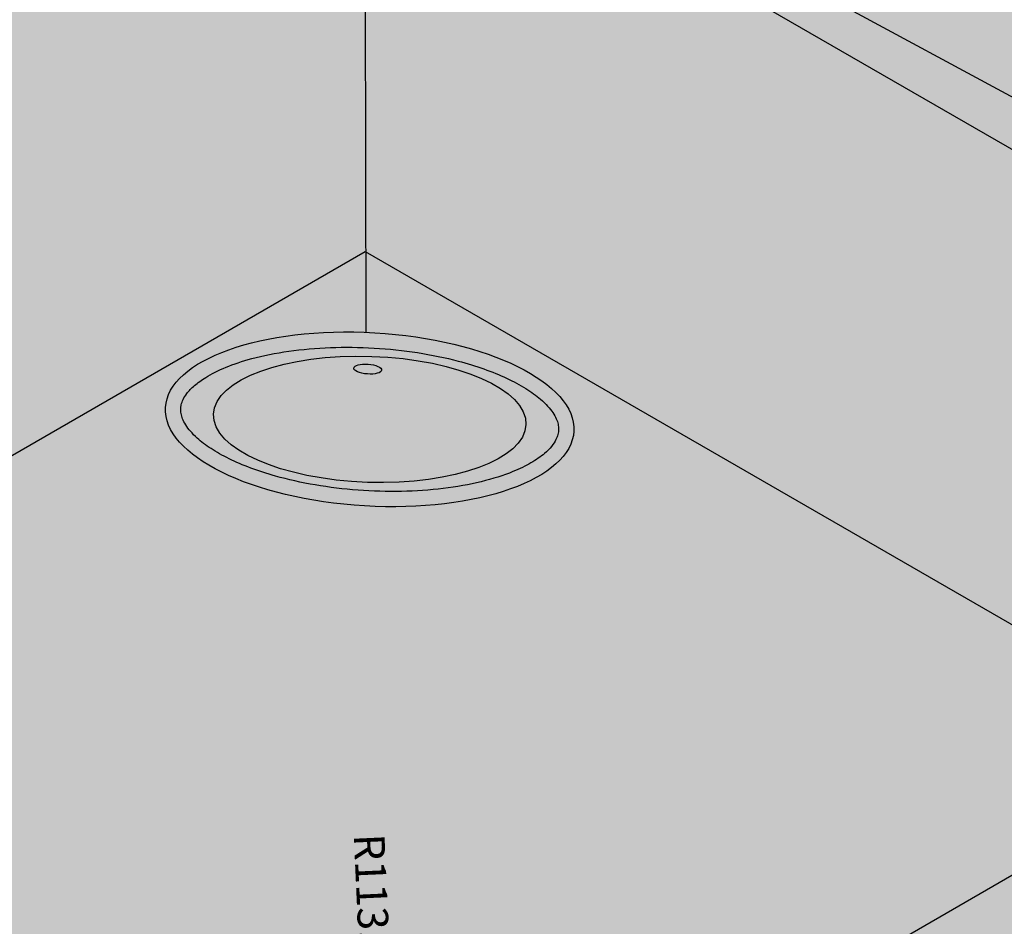
# Model space of a CAD drawing. Units: millimetres. Extents: x 78378 to 86415, y 148682 to 152721.
# Tile 13 of 18: x 80164 to 80806, y 150495 to 151086. Entities that reach past the tile are written whole.
import ezdxf

# ---------------------------------------------------------------- set-up
doc = ezdxf.new("R2010")
doc.units = ezdxf.units.MM
for name, color, linetype, lineweight in [('A-ANNO-DIMS', 2, 'Continuous', 18), ('A-FURN', 4, 'Continuous', 25), ('A-FURN-PATT', 32, 'Continuous', 13)]:
    doc.layers.add(name, color=color, linetype=linetype, lineweight=lineweight)
doc.styles.get("Standard").update_dxf_attribs({"font": 'arial.ttf'})
doc.dimstyles.new('ISO-25', dxfattribs={"dimtxt": 20, "dimasz": 20, "dimexe": 1.25, "dimexo": 0.625, "dimtad": 0, "dimdec": 1, "dimtxsty": 'Standard', "dimcen": 2.5, "dimadec": 0, "dimazin": 0, "dimtfac": 1, "dimtdec": 1, "dimtmove": 0, "dimatfit": 3, "dimfxl": 1, "dimarcsym": 0})

# ---------------------------------------------------------------- blocks, each defined once
blk = doc.blocks.new('*D65')
at = {"layer": 'A-ANNO-DIMS', "color": 0, "lineweight": -2, "transparency": 16777216}
for p, q in [((80394.08, 150453.29), (80394.98, 150433.31)), ((80401.02, 150300.38), (80395.89, 150413.33))]:
    blk.add_line(p, q, dxfattribs=at)
at = {"layer": 'A-ANNO-DIMS', "color": 0, "transparency": 16777216}
blk.add_solid([(80398.31, 150433.46), (80391.65, 150433.16), (80395.89, 150413.33)], dxfattribs=at)
at = {"layer": 'Defpoints', "color": 0, "transparency": 16777216}
for p in [(80395.89, 150413.33), (80401.02, 150300.38)]:
    blk.add_point(p, dxfattribs=at)
at = {"layer": 'A-ANNO-DIMS', "color": 0, "transparency": 16777216, "insert": (80391.73, 150504.94), "char_height": 20, "attachment_point": 5, "rotation": 272.60064}
blk.add_mtext('R113.06', dxfattribs=at)

msp = doc.modelspace()

# ---------------------------------------------------------------- hatches: boundary and pattern name
at = {"layer": 'A-FURN-PATT'}
h = msp.add_hatch(color=256, dxfattribs=at)
h.dxf.hatch_style = 1
h.paths.add_polyline_path([(78839.3276, 151040.0076), (78579.52, 151190.0076), (78579.52, 150470.0076), (78839.3276, 150320.0076)])
h.paths.add_polyline_path([(79073.1545, 150899.6469, 0.27777969), (79002.2645, 150996.3205, 0.79108393), (78917.9567, 150978.8719, 0.18044832), (78856.6481, 150853.0138), (78856.6481, 150350.6973), (79073.1545, 150484.318)])
h.paths.add_polyline_path([(79073.1545, 151175.0076), (78856.6481, 151050.0076), (78856.6481, 150853.0138, -0.18044832), (78917.9567, 150978.8719, -0.79108393), (79002.2645, 150996.3205, -0.27777969), (79073.1545, 150899.6469)])
h.paths.add_polyline_path([(79341.6224, 151350.0076), (79099.1352, 151490.0076), (78596.8405, 151200.0076), (78839.3276, 151060.0076)])
h.paths.add_polyline_path([(79904.5389, 151675.0076), (79662.0518, 151815.0076), (79099.1352, 151490.0076), (79341.6224, 151350.0076)])
h.paths.add_polyline_path([(80389.5131, 151955.0076), (80389.5131, 152235.0076), (79662.0518, 151815.0076), (79904.5389, 151675.0076)])
h.paths.add_polyline_path([(80389.5131, 151955.0076), (80164.3465, 151825.0076), (80164.3465, 151105.0076), (80614.6797, 151105.0076), (80614.6797, 151825.0076)])
edge = h.paths.add_edge_path(flags=16)
edge.add_spline(control_points=[(80216.308, 151728.251), (80227.1854, 151732.981), (80256.3301, 151745.6544), (80298.41, 151761.9595), (80340.2597, 151805.855), (80391.0771, 151782.0404), (80454.0396, 151805.7581), (80496.5007, 151742.4095), (80543.8218, 151733.4043), (80562.7182, 151729.8083)], knot_values=[0, 0, 0, 0, 35.54374676, 95.23575347, 136.36767513, 200.93298197, 236.72641081, 322.88993498, 380.17027367, 380.17027367, 380.17027367, 380.17027367], degree=3, periodic=0)
edge.add_line((80562.7182, 151729.8083), (80562.7182, 151165.0076))
edge.add_line((80562.7182, 151165.0076), (80216.308, 151165.0076))
edge.add_line((80216.308, 151165.0076), (80216.308, 151728.251))
h.paths.add_polyline_path([(80632.0002, 152095.0076), (80389.5131, 152235.0076), (80389.5131, 151955.0076), (80614.6797, 151825.0076), (80632.0002, 151815.0076)])
h.paths.add_polyline_path([(80867.7794, 151958.8805), (80632.0002, 152095.0076), (80632.0002, 151815.0076), (80632.0002, 151510.0076), (80867.7794, 151373.8805)])
h.paths.add_polyline_path([(80147.026, 151495.8203, 0.18918979), (80063.5671, 151597.7244, 0.78826136), (79979.2691, 151580.5832, 0.16072613), (79904.5389, 151413.5769), (79904.5389, 150955.0076), (80147.026, 151095.0076)])
h.paths.add_polyline_path([(80147.026, 151815.0076), (79904.5389, 151675.0076), (79904.5389, 151413.5769, -0.16072613), (79979.2691, 151580.5832, -0.78826136), (80063.5671, 151597.7244, -0.18918979), (80147.026, 151495.8203)])
h.paths.add_polyline_path([(79887.2184, 151645.0076), (79640.4011, 151502.5076), (79640.4011, 151262.3325, -0.16072613), (79715.1313, 151429.3387, -0.78826136), (79799.4294, 151446.48, -0.21290578), (79887.2184, 151328.7247)])
h.paths.add_polyline_path([(79799.4294, 151446.48, 0.78826136), (79715.1313, 151429.3387, 0.16072613), (79640.4011, 151262.3325), (79640.4011, 150822.5076), (79887.2184, 150965.0076), (79887.2184, 151328.7247, 0.21290578)])
h.paths.add_polyline_path([(79605.7601, 151482.5076), (79358.9429, 151340.0076), (79358.9429, 151100.0701, -0.16072613), (79433.6731, 151267.0764, -0.78826136), (79517.9711, 151284.2176, -0.21290578), (79605.7601, 151166.4623)])
h.paths.add_polyline_path([(79605.7601, 151166.4623, 0.21290578), (79517.9711, 151284.2176, 0.78826136), (79433.6731, 151267.0764, 0.16072613), (79358.9429, 151100.0701), (79358.9429, 150742.9831), (79419.0877, 150694.7323), (79605.7601, 150802.5076)])
edge = h.paths.add_edge_path(flags=0)
edge.add_spline(control_points=[(81152.4356, 151098.7676), (81105.7208, 151145.9466), (81038.6136, 151213.7208), (80882.3866, 151214.1938), (80797.4434, 151311.2997), (80711.8686, 151340.3754), (80681.7691, 151350.6023)], knot_values=[0, 0, 0, 0, 188.233441, 270.4032752, 445.45179201, 540.42858829, 540.42858829, 540.42858829, 540.42858829], degree=3, periodic=0)
edge.add_line((80683.4538, 151350.0269), (80683.4538, 151104.8792))
edge.add_line((80683.4538, 151104.8792), (81152.4356, 150851.399))
edge.add_line((81152.4356, 150851.399), (81152.4356, 151098.7676))
edge = h.paths.add_edge_path(flags=0)
edge.add_spline(control_points=[(80912.9018, 151027.1103), (80892.3742, 151034.1027), (80860.1663, 151045.0739), (80835.5097, 151068.1214), (80826.5679, 151076.4797)], knot_values=[0, 0, 0, 0, 63.98405104, 100.39142428, 100.39142428, 100.39142428, 100.39142428], degree=3, periodic=0)
edge.add_arc((80830.0414, 151081.2992), 5.9407, 100.9277276, 234.2187381, ccw=False)
edge.add_spline(control_points=[(80828.9152, 151087.1322), (80837.857, 151078.7739), (80862.5136, 151055.7263), (80894.7215, 151044.7552), (80915.2491, 151037.7628)], knot_values=[0, 0, 0, 0, 36.40737324, 100.39142428, 100.39142428, 100.39142428, 100.39142428], degree=3, periodic=0)
edge.add_arc((80914.7882, 151032.2795), 5.5026, -107.9540399, 85.195579, ccw=False)
h.paths.add_polyline_path([(81238.218, 151110.0076), (80632.0002, 151460.0076), (80632.0002, 151105.0076), (81238.218, 150755.0076)])
edge = h.paths.add_edge_path(flags=16)
edge.add_line((81152.4356, 150851.399), (80683.4538, 151104.8792))
edge.add_line((80683.4538, 151104.8792), (80683.4538, 151350.0279))
edge.add_spline(control_points=[(80681.7691, 151350.6023), (80711.8686, 151340.3754), (80797.4434, 151311.2997), (80882.3866, 151214.1938), (81038.6136, 151213.7208), (81105.7208, 151145.9466), (81152.4356, 151098.7676)], knot_values=[0, 0, 0, 0, 94.97679628, 270.02531309, 352.19514729, 540.42858829, 540.42858829, 540.42858829, 540.42858829], degree=3, periodic=0)
edge.add_line((81152.4356, 151098.7676), (81152.4356, 150851.399))
edge = h.paths.add_edge_path(flags=0)
edge.add_spline(control_points=[(80912.9018, 151027.1103), (80892.3742, 151034.1027), (80860.1663, 151045.0739), (80835.5097, 151068.1214), (80826.5679, 151076.4797)], knot_values=[0, 0, 0, 0, 63.98405104, 100.39142428, 100.39142428, 100.39142428, 100.39142428], degree=3, periodic=0)
edge.add_arc((80830.0414, 151081.2992), 5.9407, 100.9277276, 234.2187381, ccw=False)
edge.add_spline(control_points=[(80828.9152, 151087.1322), (80837.857, 151078.7739), (80862.5136, 151055.7263), (80894.7215, 151044.7552), (80915.2491, 151037.7628)], knot_values=[0, 0, 0, 0, 36.40737324, 100.39142428, 100.39142428, 100.39142428, 100.39142428], degree=3, periodic=0)
edge.add_arc((80914.7882, 151032.2795), 5.5026, -107.7417882, 85.195579, ccw=False)
h.paths.add_polyline_path([(81498.0256, 151255.0076), (81238.218, 151110.0076), (81238.218, 150755.0076), (81498.0256, 150905.0076)])
edge = h.paths.add_edge_path(flags=16)
edge.add_spline(control_points=[(81152.4356, 151098.7676), (81105.7208, 151145.9466), (81038.6136, 151213.7208), (80882.3866, 151214.1938), (80797.4434, 151311.2997), (80711.8686, 151340.3754), (80681.7691, 151350.6023)], knot_values=[0, 0, 0, 0, 188.233441, 270.4032752, 445.45179201, 540.42858829, 540.42858829, 540.42858829, 540.42858829], degree=3, periodic=0)
edge.add_line((80683.4538, 151350.0279), (80683.4538, 151104.8792))
edge.add_line((80683.4538, 151104.8792), (81152.4356, 150851.399))
edge.add_line((81152.4356, 150851.399), (81152.4356, 151098.7676))
h.paths.add_polyline_path([(81453.9904, 151280.4314), (80867.7794, 151618.8805), (80867.7794, 151373.8805), (81238.218, 151160.0076)])
edge = h.paths.add_edge_path(flags=16)
edge.add_line((81189.2304, 151297.6373), (81114.4166, 151300.2154))
edge.add_arc((81412.0967, 151394.0167), 312.1092, 179.7569303, 197.4900342, ccw=False)
edge.add_ellipse((81154.0183, 151392.0436), major_axis=(-54.0264, 3.6301), ratio=0.22179693, start_angle=0, end_angle=0.3517985, ccw=False)
edge.add_ellipse((81154.0183, 151392.0436), major_axis=(-54.0264, 3.6301), ratio=0.22179693, start_angle=180, end_angle=360, ccw=False)
edge.add_spline(control_points=[(81196.1844, 151321.9476), (81224.9802, 151347.1455), (81266.8846, 151383.8144), (81222.0354, 151387.0304), (81208.0056, 151388.0364)], knot_values=[0, 0, 0, 0, 75.09175173, 109.27580439, 109.27580439, 109.27580439, 109.27580439], degree=3, periodic=0)
edge.add_arc((80751.9112, 151435.6145), 458.5693, 342.4891602, 345.646172, ccw=False)
edge = h.paths.add_edge_path(flags=0)
edge.add_spline(control_points=[(81196.6193, 151323.657), (81197.893, 151324.7717), (81199.1654, 151325.8858), (81209.0233, 151334.5343), (81217.3959, 151341.9835), (81228.0928, 151352.5012), (81231.3883, 151355.9524), (81236.9493, 151362.4395), (81239.214, 151365.4773), (81241.4987, 151369.416), (81242.064, 151370.5542), (81242.9187, 151372.6971), (81243.2076, 151373.7015), (81243.5012, 151375.5539), (81243.5065, 151376.4), (81243.2432, 151377.9407), (81242.9775, 151378.6373), (81242.1402, 151379.937), (81241.5659, 151380.5416), (81240.2039, 151381.533), (81239.4963, 151381.9384), (81237.0619, 151383.0663), (81235.0242, 151383.6999), (81230.352, 151384.7569), (81227.7173, 151385.1826), (81221.9118, 151385.9145), (81218.7193, 151386.2133), (81213.7912, 151386.6115), (81212.1252, 151386.7359), (81209.6196, 151386.9181), (81208.7865, 151386.9779), (81207.9009, 151387.0432)], knot_values=[0.01548744, 0.01548744, 0.01548744, 0.01548744, 3.33787957, 3.33787957, 25.85130624, 25.85130624, 37.52811308, 37.52811308, 49.20491992, 49.20491992, 54.2850938, 54.2850938, 59.36526768, 59.36526768, 64.44544157, 64.44544157, 69.52561545, 69.52561545, 74.60578933, 74.60578933, 78.49366785, 78.49366785, 86.25567095, 86.25567095, 94.01767406, 94.01767406, 102.20226556, 102.20226556, 106.29456131, 106.29456131, 108.32522175, 108.32522175, 108.32522175, 108.32522175], degree=3, periodic=0)
edge = h.paths.add_edge_path(flags=16)
edge.add_arc((81034.1732, 151350.4693), 42.5822, 231.2679035, 306.151846, ccw=False)
edge.add_line((81007.5303, 151317.2517), (81007.5303, 151395.181))
edge.add_ellipse((81033.412, 151394.7791), major_axis=(-25.8816, 0.4538), ratio=0.23894509, start_angle=0, end_angle=0.1147075, ccw=False)
edge.add_ellipse((81033.412, 151394.7791), major_axis=(-25.8816, 0.4538), ratio=0.23894509, start_angle=181.1677709, end_angle=358.9476457, ccw=False)
edge.add_ellipse((81033.412, 151395.7791), major_axis=(-25.8816, 0.4538), ratio=0.23894509, start_angle=180, end_angle=360.1147075, ccw=False)
edge.add_ellipse((81033.412, 151395.7791), major_axis=(-25.8816, 0.4538), ratio=0.23894509, start_angle=178.9476457, end_angle=180, ccw=False)
edge.add_line((81059.2936, 151395.1778), (81059.2936, 151394.3772))
edge.add_ellipse((81033.412, 151394.7791), major_axis=(-25.8816, 0.4538), ratio=0.23894509, start_angle=180, end_angle=180.1147075, ccw=False)
edge.add_ellipse((81033.412, 151394.7791), major_axis=(-25.8816, 0.4538), ratio=0.23894509, start_angle=3.6903098, end_angle=176.4406503, ccw=False)
edge.add_line((81059.2936, 151393.3388), (81059.2936, 151316.086))
h.paths.add_polyline_path([(80951.9355, 151343.9568), (80909.6838, 151362.4635), (80904.0219, 151443.9615, -0.38133308), (80987.2169, 151411.3717)], flags=16)
h = msp.add_hatch(color=256, dxfattribs=at)
h.dxf.hatch_style = 1
h.paths.add_polyline_path([(80389.8136, 150935.1811), (80389.5131, 151105.0076), (80164.3465, 151105.0076), (79904.5389, 150955.0076), (79433.5848, 150683.1022), (79459.4128, 150662.3818), (79243.9048, 150537.9582), (79160.4069, 150518.1674), (78839.3276, 150320.0076), (78579.52, 150470.0076), (78570.8597, 150475.0076), (78570.8597, 150465.0076), (78570.8597, 149885.0076)])
h.paths.add_polyline_path([(80086.4042, 150460.0076), (79826.5966, 150610.0076), (78570.8597, 149885.0076), (78830.6674, 149735.0076)])
h.paths.add_polyline_path([(79540.8001, 150161.0557), (79217.3967, 149974.3386), (78980.9166, 150110.8705), (79304.32, 150297.5875)], flags=16)
h.paths.add_polyline_path([(79506.159, 150161.0557), (79217.3967, 149994.3386), (79015.5576, 150110.8705), (79304.32, 150277.5875)], flags=0)
edge = h.paths.add_edge_path(flags=0)
edge.add_arc((79247.8636, 150177.1541), 137.9799, 256.0025928, 293.5594109)
edge.add_arc((79240.7671, 150078.2605), 68.0855, 336.099104, 387.3696877)
edge.add_ellipse((79258.3074, 150109.4852), major_axis=(-42.6234, -1.6591), ratio=0.16042843, start_angle=0, end_angle=179.0977279, ccw=False)
edge.add_arc((79285.2112, 150074.2509), 77.2096, 155.1233104, 203.6557939)
edge = h.paths.add_edge_path(flags=0)
edge.add_ellipse((79258.6958, 150110.8297), major_axis=(-42.6234, -1.6591), ratio=0.16042843, start_angle=350.6039412, end_angle=356.2289762)
edge.add_line((79219.169, 150111.8937), (79218.3268, 150109.4141))
edge.add_arc((79262.4675, 150032.9602), 88.2813, 112.3931229, 120, ccw=False)
h.paths.add_polyline_path([(79287.0625, 150086.9703, -0.24770206), (79288.1967, 150077.2955, -0.39047651), (79265.4731, 150072.5438, -0.48726153), (79264.079, 150082.3769, 0.39560433)], flags=0)
h.paths.add_polyline_path([(80389.5131, 150935.0076), (79826.5966, 150610.0076), (80086.4042, 150460.0076), (80692.622, 150460.0076), (80952.4296, 150610.0076)])
edge = h.paths.add_edge_path(flags=16)
edge.add_ellipse((80392.4466, 150825.601), major_axis=(-133.0757, 7.722), ratio=0.42449957, start_angle=0, end_angle=360)
edge = h.paths.add_edge_path(flags=0)
edge.add_spline(control_points=[(80269.3541, 150832.7436), (80269.2919, 150831.672), (80269.3503, 150830.5922), (80269.7341, 150828.3361), (80270.0612, 150827.1587), (80271.0461, 150824.6748), (80271.7052, 150823.3692), (80273.4061, 150820.6503), (80274.4481, 150819.2381), (80276.9366, 150816.3509), (80278.3828, 150814.8762), (80282.5858, 150811.0913), (80285.6261, 150808.7701), (80292.6031, 150804.2267), (80296.5388, 150802.0041), (80305.195, 150797.7581), (80309.9151, 150795.7344), (80320.0112, 150791.96), (80325.387, 150790.2092), (80339.2162, 150786.315), (80347.9578, 150784.3563), (80366.0679, 150781.2568), (80375.4359, 150780.1158), (80394.3093, 150778.7158), (80403.8142, 150778.4568), (80422.4656, 150778.8319), (80431.6115, 150779.4662), (80449.0608, 150781.5838), (80457.3636, 150783.0675), (80472.6699, 150786.7766), (80479.6726, 150789.0033), (80490.1894, 150793.2813), (80494.1268, 150795.1967), (80501.0146, 150799.1885), (80503.9632, 150801.2651), (80508.2066, 150804.9015), (80509.73, 150806.4609), (80512.1996, 150809.4942), (80513.1456, 150810.9657), (80514.4291, 150813.5431), (80514.8436, 150814.6688), (80515.3984, 150816.8625), (80515.5405, 150817.9315), (80515.5801, 150820.098), (80515.4773, 150821.1978), (80514.9905, 150823.5062), (80514.6047, 150824.7154), (80513.4854, 150827.2641), (80512.7511, 150828.6027), (80510.8872, 150831.3809), (80509.7578, 150832.8196), (80507.0873, 150835.7513), (80505.5466, 150837.2439), (80501.0624, 150841.0944), (80497.8199, 150843.4576), (80490.4174, 150848.062), (80486.2582, 150850.3037), (80477.1448, 150854.5643), (80472.1909, 150856.5835), (80461.6275, 150860.3245), (80456.0182, 150862.0465), (80441.7332, 150865.8127), (80432.7885, 150867.6675), (80414.3391, 150870.5317), (80404.8349, 150871.5411), (80385.7707, 150872.6572), (80376.2113, 150872.764), (80357.5444, 150872.0728), (80348.4375, 150871.2748), (80331.1682, 150868.83), (80323.0064, 150867.1827), (80309.472, 150863.5363), (80303.8628, 150861.6593), (80293.8018, 150857.5401), (80289.3512, 150855.2969), (80282.7757, 150851.2345), (80280.3473, 150849.4579), (80276.2606, 150845.9127), (80274.604, 150844.1458), (80272.3157, 150841.1243), (80271.5358, 150839.8454), (80270.3496, 150837.3879), (80269.9417, 150836.2101), (80269.5065, 150834.2815), (80269.3988, 150833.5143), (80269.3541, 150832.7436)], knot_values=[0, 0, 0, 0, 0.09750046, 0.09750046, 0.19500092, 0.19500092, 0.29250138, 0.29250138, 0.39000184, 0.39000184, 0.4875023, 0.4875023, 0.63880322, 0.63880322, 0.79010415, 0.79010415, 0.94140507, 0.94140507, 1.092706, 1.092706, 1.3128171, 1.3128171, 1.5329282, 1.5329282, 1.7530393, 1.7530393, 1.97315041, 1.97315041, 2.19326151, 2.19326151, 2.41337261, 2.41337261, 2.56986063, 2.56986063, 2.72634866, 2.72634866, 2.84418658, 2.84418658, 2.96202451, 2.96202451, 3.06023388, 3.06023388, 3.15844325, 3.15844325, 3.25665261, 3.25665261, 3.35486198, 3.35486198, 3.45307135, 3.45307135, 3.55128072, 3.55128072, 3.64949009, 3.64949009, 3.80392773, 3.80392773, 3.95836537, 3.95836537, 4.11280301, 4.11280301, 4.26724064, 4.26724064, 4.48920349, 4.48920349, 4.71116635, 4.71116635, 4.9331292, 4.9331292, 5.15509205, 5.15509205, 5.3770549, 5.3770549, 5.55785361, 5.55785361, 5.73865232, 5.73865232, 5.87239556, 5.87239556, 6.00613879, 6.00613879, 6.109605, 6.109605, 6.2130712, 6.2130712, 6.28318531, 6.28318531, 6.28318531, 6.28318531], degree=3, periodic=0)
edge = h.paths.add_edge_path(flags=0)
edge.add_ellipse((80392.4466, 150825.601), major_axis=(-101.8398, 3.3923), ratio=0.40349248, start_angle=0, end_angle=360)
edge = h.paths.add_edge_path(flags=0)
edge.add_ellipse((80391.1657, 150858.3746), major_axis=(9.0882, -0.6733), ratio=0.35135413, start_angle=0, end_angle=360)
h.paths.add_polyline_path([(80952.4296, 150610.0076), (80692.622, 150460.0076), (81361.2342, 150073.9842), (81649.9628, 150052.7286), (81766.4935, 150120.0076), (81766.4935, 150140.0076), (81564.9025, 150256.3963), (81564.8884, 150096.1963), (81538.9076, 150111.1963), (81538.9217, 150271.3963)])
h.paths.add_polyline_path([(81539.0357, 151571.3305), (80867.7794, 151958.8805), (80867.7794, 151618.8805), (81498.0256, 151255.0076), (81498.0256, 150905.0076), (81238.218, 150755.0076), (81538.9488, 150581.3806)])
h.paths.add_polyline_path([(81766.4935, 151440.0076), (81565.0164, 151556.3305), (81564.9296, 150566.3806), (81766.4935, 150450.0076)])
edge = h.paths.add_edge_path()
edge.add_line((81564.9296, 150566.3806), (81564.9137, 150384.6289))
edge.add_ellipse((81552.1304, 150358.5718), major_axis=(52.6272, 3.506), ratio=0.49589905, start_angle=367.5169757, end_angle=420.0564686, ccw=False)
edge.add_ellipse((81552.1304, 150358.5718), major_axis=(52.6272, 3.506), ratio=0.49589905, start_angle=351.729742, end_angle=367.5169757, ccw=False)
edge.add_ellipse((81552.1304, 150345.5016), major_axis=(52.6272, 3.506), ratio=0.49589905, start_angle=352.5116949, end_angle=366.3006092, ccw=False)
edge.add_line((81603.4463, 150342.2039), (81603.5064, 150340.4475))
edge.add_ellipse((81552.1304, 150332.128), major_axis=(52.6272, 3.506), ratio=0.49589905, start_angle=353.6729654, end_angle=365.3867997, ccw=False)
edge.add_ellipse((81552.1304, 150332.128), major_axis=(52.6272, 3.506), ratio=0.49589905, start_angle=350.9388331, end_angle=353.6729654)
edge.add_line((81603.8688, 150329.855), (81604.0442, 150324.7302))
edge.add_ellipse((81552.1304, 150317.7418), major_axis=(52.6272, 3.506), ratio=0.49589905, start_angle=355.2176746, end_angle=363.8553364, ccw=False)
edge.add_ellipse((81552.1304, 150317.7418), major_axis=(52.6272, 3.506), ratio=0.49589905, start_angle=341.3250873, end_angle=355.2176746, ccw=False)
edge.add_ellipse((81552.1304, 150317.7418), major_axis=(52.6272, 3.506), ratio=0.49589905, start_angle=293.4661701, end_angle=341.3250873, ccw=False)
edge.add_line((81564.9057, 150292.9664), (81564.9025, 150256.3963))
edge.add_line((81564.9025, 150256.3963), (81766.4935, 150140.0076))
edge.add_line((81766.4935, 150140.0076), (81766.4935, 150450.0076))
edge.add_line((81766.4935, 150450.0076), (81564.9296, 150566.3806))
h.paths.add_polyline_path([(81525.5713, 150321.598), (81526.5985, 150321.3069), (81528.6771, 150320.947)])
h.paths.add_polyline_path([(81512.7903, 150326.1129), (81514.5058, 150325.3887), (81512.538, 150326.2678)])
h.paths.add_polyline_path([(81533.2148, 150320.1615), (81534.6952, 150319.9052), (81536.5995, 150319.7557)])
h.paths.add_polyline_path([(81518.622, 150323.6513), (81519.227, 150323.3959), (81521.289, 150322.8116)])
h.paths.add_polyline_path([(81501.2183, 150336.2599), (81500.3543, 150338.1339), (81499.7815, 150340.0494), (81499.5032, 150341.9955), (81499.5032, 150343.7257), (81499.7584, 150345.5905), (81500.2766, 150347.4549), (81501.0551, 150349.3095), (81501.0967, 150349.3937), (81501.1389, 150349.4778), (81500.9978, 150349.7496), (81500.8628, 150350.0225), (81499.5032, 150355.0658), (81499.9591, 150359.5002), (81501.8982, 150363.9083), (81505.2653, 150368.1646), (81509.9647, 150372.1482), (81515.8627, 150375.7459), (81522.7918, 150378.8553), (81530.555, 150381.3882), (81538.9315, 150383.2724), (81538.9488, 150581.3806), (80632.0002, 151105.0076), (80389.5131, 151105.0076), (80389.8142, 150934.8338), (80952.4296, 150610.0076), (81538.9217, 150271.3963), (81538.9234, 150291.7194), (81538.8752, 150291.721), (81530.1915, 150292.8239), (81522.1802, 150294.6904), (81515.0866, 150297.2633), (81509.8635, 150299.9959), (81505.6084, 150303.1351), (81502.419, 150306.6088), (81500.3683, 150310.3375), (81499.5032, 150314.2358), (81499.5032, 150315.9659), (81499.8206, 150318.1159), (81500.487, 150320.2634), (81501.4979, 150322.3941), (81500.487, 150324.4233), (81499.8206, 150326.5039), (81499.5032, 150328.622), (81499.5032, 150330.3521), (81499.7815, 150332.3262), (81500.3543, 150334.2992)])
h = msp.add_hatch(color=256, dxfattribs=at)
h.dxf.hatch_style = 1
h.paths.add_polyline_path([(79090.475, 151205.0076), (78839.3276, 151060.0076), (78839.3276, 150320.0076), (79090.475, 150475.0076)])
h.paths.add_polyline_path([(79073.1545, 151175.0076), (79073.1545, 150899.6469, -0.04544363), (79073.1545, 150878.5653), (79073.1545, 150484.318), (78856.6481, 150350.6973), (78856.6481, 150814.5249, -0.04815716), (78856.6481, 150853.0138), (78856.6481, 151050.0076)], flags=16)
h.paths.add_polyline_path([(79358.9429, 151340.0076), (79605.7601, 151482.5076), (79605.7601, 150802.5076), (79419.0877, 150694.7323), (79433.5848, 150683.1022), (79623.0806, 150792.5076), (79623.0806, 151512.5076), (79341.6224, 151350.0076), (79341.6224, 150756.8784), (79358.9429, 150742.9831)])
h.paths.add_polyline_path([(79341.6224, 151350.0076), (79090.475, 151205.0076), (79090.475, 150475.0076), (79160.4069, 150518.1674), (79107.7955, 150505.6973), (79107.7955, 151195.0076), (79109.5275, 151196.0076), (79324.3018, 151320.0076), (79324.3018, 150770.7736), (79341.6224, 150756.8784)])
h.paths.add_polyline_path([(79887.2184, 151645.0076), (79887.2184, 151665.0076), (79623.0806, 151512.5076), (79623.0806, 150792.5076), (79887.2184, 150945.0076), (79887.2184, 150965.0076), (79640.4011, 150822.5076), (79640.4011, 151502.5076)])
h.paths.add_polyline_path([(79904.5389, 151655.0076), (79887.2184, 151645.0076), (79887.2184, 150965.0076), (79904.5389, 150975.0076)])
h.paths.add_polyline_path([(80164.3465, 151825.0076), (80147.026, 151815.0076), (80147.026, 151095.0076), (80164.3465, 151105.0076)])
h.paths.add_polyline_path([(80632.0002, 151510.0076), (80632.0002, 151490.0076), (81238.218, 151140.0076), (81471.6045, 151270.2619), (81453.9904, 151280.4314), (81238.218, 151160.0076)])
h.paths.add_polyline_path([(80632.0002, 151490.0076), (80632.0002, 151470.0076), (81238.218, 151120.0076), (81489.2186, 151260.0924), (81471.6045, 151270.2619), (81238.218, 151140.0076)])
h.paths.add_polyline_path([(80632.0002, 151460.0076), (80632.0002, 151105.0076), (81238.218, 150755.0076), (81238.218, 151110.0076)])
edge = h.paths.add_edge_path(flags=16)
edge.add_spline(control_points=[(80681.7691, 151350.6023), (80711.8686, 151340.3754), (80797.4434, 151311.2997), (80882.3866, 151214.1938), (81038.6136, 151213.7208), (81105.7208, 151145.9466), (81152.4356, 151098.7676)], knot_values=[0, 0, 0, 0, 94.97679628, 270.02531309, 352.19514729, 540.42858829, 540.42858829, 540.42858829, 540.42858829], degree=3, periodic=0)
edge.add_line((81152.4356, 151098.7676), (81152.4356, 150851.399))
edge.add_line((81152.4356, 150851.399), (80683.4538, 151104.8792))
edge.add_line((80683.4538, 151104.8792), (80683.4538, 151350.027))
edge = h.paths.add_edge_path(flags=0)
edge.add_spline(control_points=[(80828.9152, 151087.1322), (80837.857, 151078.7739), (80862.5136, 151055.7263), (80894.7215, 151044.7552), (80915.2491, 151037.7628)], knot_values=[0, 0, 0, 0, 36.40737324, 100.39142428, 100.39142428, 100.39142428, 100.39142428], degree=3, periodic=0)
edge.add_arc((80914.7882, 151032.2795), 5.5026, -107.9540399, 85.195579, ccw=False)
edge.add_spline(control_points=[(80912.9018, 151027.1103), (80892.3742, 151034.1027), (80860.1663, 151045.0739), (80835.5097, 151068.1214), (80826.5679, 151076.4797)], knot_values=[0, 0, 0, 0, 63.98405104, 100.39142428, 100.39142428, 100.39142428, 100.39142428], degree=3, periodic=0)
edge.add_arc((80830.0414, 151081.2992), 5.9407, 100.9277276, 234.2187381, ccw=False)
h.paths.add_polyline_path([(80632.0002, 151815.0076), (80614.6797, 151825.0076), (80614.6797, 151105.0076), (80632.0002, 151105.0076)])
h.paths.add_polyline_path([(81498.0256, 151255.0076), (81489.2186, 151260.0924), (81238.218, 151120.0076), (80632.0002, 151470.0076), (80632.0002, 151460.0076), (81238.218, 151110.0076)])
h.paths.add_polyline_path([(78596.8405, 151200.0076), (78579.52, 151190.0076), (78839.3276, 151040.0076), (78839.3276, 151060.0076)])
h.paths.add_polyline_path([(78596.8405, 151200.0076), (78579.52, 151210.0076), (78579.52, 151190.0076)])
h.paths.add_polyline_path([(78579.52, 151210.0076), (78570.8597, 151205.0076), (78570.8597, 150475.0076), (78579.52, 150470.0076)])
h = msp.add_hatch(color=256, dxfattribs=at)
h.dxf.hatch_style = 1
edge = h.paths.add_edge_path()
edge.add_ellipse((80392.4466, 150825.601), major_axis=(-133.0757, 7.722), ratio=0.42449957, start_angle=0, end_angle=275.8822062)
edge.add_ellipse((80392.4466, 150825.601), major_axis=(-133.0757, 7.722), ratio=0.42449957, start_angle=275.8822062, end_angle=360)
edge = h.paths.add_edge_path(flags=16)
edge.add_spline(control_points=[(80269.3541, 150832.7436), (80269.2919, 150831.672), (80269.3503, 150830.5922), (80269.7341, 150828.3361), (80270.0612, 150827.1587), (80271.0461, 150824.6748), (80271.7052, 150823.3692), (80273.4061, 150820.6503), (80274.4481, 150819.2381), (80276.9366, 150816.3509), (80278.3828, 150814.8762), (80282.5858, 150811.0913), (80285.6261, 150808.7701), (80292.6031, 150804.2267), (80296.5388, 150802.0041), (80305.195, 150797.7581), (80309.9151, 150795.7344), (80320.0112, 150791.96), (80325.387, 150790.2092), (80339.2162, 150786.315), (80347.9578, 150784.3563), (80366.0679, 150781.2568), (80375.4359, 150780.1158), (80394.3093, 150778.7158), (80403.8142, 150778.4568), (80422.4656, 150778.8319), (80431.6115, 150779.4662), (80449.0608, 150781.5838), (80457.3636, 150783.0675), (80472.6699, 150786.7766), (80479.6726, 150789.0033), (80490.1894, 150793.2813), (80494.1268, 150795.1967), (80501.0146, 150799.1885), (80503.9632, 150801.2651), (80508.2066, 150804.9015), (80509.73, 150806.4609), (80512.1996, 150809.4942), (80513.1456, 150810.9657), (80514.4291, 150813.5431), (80514.8436, 150814.6688), (80515.3984, 150816.8625), (80515.5405, 150817.9315), (80515.5801, 150820.098), (80515.4773, 150821.1978), (80514.9905, 150823.5062), (80514.6047, 150824.7154), (80513.4854, 150827.2641), (80512.7511, 150828.6027), (80510.8872, 150831.3809), (80509.7578, 150832.8196), (80507.0873, 150835.7513), (80505.5466, 150837.2439), (80501.0624, 150841.0944), (80497.8199, 150843.4576), (80490.4174, 150848.062), (80486.2582, 150850.3037), (80477.1448, 150854.5643), (80472.1909, 150856.5835), (80461.6275, 150860.3245), (80456.0182, 150862.0465), (80441.7332, 150865.8127), (80432.7885, 150867.6675), (80414.3391, 150870.5317), (80404.8349, 150871.5411), (80385.7707, 150872.6572), (80376.2113, 150872.764), (80357.5444, 150872.0728), (80348.4375, 150871.2748), (80331.1682, 150868.83), (80323.0064, 150867.1827), (80309.472, 150863.5363), (80303.8628, 150861.6593), (80293.8018, 150857.5401), (80289.3512, 150855.2969), (80282.7757, 150851.2345), (80280.3473, 150849.4579), (80276.2606, 150845.9127), (80274.604, 150844.1458), (80272.3157, 150841.1243), (80271.5358, 150839.8454), (80270.3496, 150837.3879), (80269.9417, 150836.2101), (80269.5065, 150834.2815), (80269.3988, 150833.5143), (80269.3541, 150832.7436)], knot_values=[0, 0, 0, 0, 0.09750046, 0.09750046, 0.19500092, 0.19500092, 0.29250138, 0.29250138, 0.39000184, 0.39000184, 0.4875023, 0.4875023, 0.63880322, 0.63880322, 0.79010415, 0.79010415, 0.94140507, 0.94140507, 1.092706, 1.092706, 1.3128171, 1.3128171, 1.5329282, 1.5329282, 1.7530393, 1.7530393, 1.97315041, 1.97315041, 2.19326151, 2.19326151, 2.41337261, 2.41337261, 2.56986063, 2.56986063, 2.72634866, 2.72634866, 2.84418658, 2.84418658, 2.96202451, 2.96202451, 3.06023388, 3.06023388, 3.15844325, 3.15844325, 3.25665261, 3.25665261, 3.35486198, 3.35486198, 3.45307135, 3.45307135, 3.55128072, 3.55128072, 3.64949009, 3.64949009, 3.80392773, 3.80392773, 3.95836537, 3.95836537, 4.11280301, 4.11280301, 4.26724064, 4.26724064, 4.48920349, 4.48920349, 4.71116635, 4.71116635, 4.9331292, 4.9331292, 5.15509205, 5.15509205, 5.3770549, 5.3770549, 5.55785361, 5.55785361, 5.73865232, 5.73865232, 5.87239556, 5.87239556, 6.00613879, 6.00613879, 6.109605, 6.109605, 6.2130712, 6.2130712, 6.28318531, 6.28318531, 6.28318531, 6.28318531], degree=3, periodic=0)
edge = h.paths.add_edge_path(flags=0)
edge.add_ellipse((80392.4466, 150825.601), major_axis=(-101.8398, 3.3923), ratio=0.40349248, start_angle=0, end_angle=360)
edge = h.paths.add_edge_path(flags=0)
edge.add_ellipse((80391.1657, 150858.3746), major_axis=(9.0882, -0.6733), ratio=0.35135413, start_angle=0, end_angle=360)
h = msp.add_hatch(color=256, dxfattribs=at)
h.dxf.hatch_style = 1
edge = h.paths.add_edge_path(flags=0)
edge.add_ellipse((80392.4466, 150825.601), major_axis=(-101.8398, 3.3923), ratio=0.40349248, start_angle=0, end_angle=360)
edge = h.paths.add_edge_path(flags=0)
edge.add_ellipse((80391.1657, 150858.3746), major_axis=(9.0882, -0.6733), ratio=0.35135413, start_angle=0, end_angle=360)
edge = h.paths.add_edge_path()
edge.add_spline(control_points=[(80269.3541, 150832.7436), (80269.2919, 150831.672), (80269.3503, 150830.5922), (80269.7341, 150828.3361), (80270.0612, 150827.1587), (80271.0461, 150824.6748), (80271.7052, 150823.3692), (80273.4061, 150820.6503), (80274.4481, 150819.2381), (80276.9366, 150816.3509), (80278.3828, 150814.8762), (80282.5858, 150811.0913), (80285.6261, 150808.7701), (80292.6031, 150804.2267), (80296.5388, 150802.0041), (80305.195, 150797.7581), (80309.9151, 150795.7344), (80320.0112, 150791.96), (80325.387, 150790.2092), (80339.2162, 150786.315), (80347.9578, 150784.3563), (80366.0679, 150781.2568), (80375.4359, 150780.1158), (80394.3093, 150778.7158), (80403.8142, 150778.4568), (80422.4656, 150778.8319), (80431.6115, 150779.4662), (80449.0608, 150781.5838), (80457.3636, 150783.0675), (80472.6699, 150786.7766), (80479.6726, 150789.0033), (80490.1894, 150793.2813), (80494.1268, 150795.1967), (80501.0146, 150799.1885), (80503.9632, 150801.2651), (80508.2066, 150804.9015), (80509.73, 150806.4609), (80512.1996, 150809.4942), (80513.1456, 150810.9657), (80514.4291, 150813.5431), (80514.8436, 150814.6688), (80515.3984, 150816.8625), (80515.5405, 150817.9315), (80515.5801, 150820.098), (80515.4773, 150821.1978), (80514.9905, 150823.5062), (80514.6047, 150824.7154), (80513.4854, 150827.2641), (80512.7511, 150828.6027), (80510.8872, 150831.3809), (80509.7578, 150832.8196), (80507.0873, 150835.7513), (80505.5466, 150837.2439), (80501.0624, 150841.0944), (80497.8199, 150843.4576), (80490.4174, 150848.062), (80486.2582, 150850.3037), (80477.1448, 150854.5643), (80472.1909, 150856.5835), (80461.6275, 150860.3245), (80456.0182, 150862.0465), (80441.7332, 150865.8127), (80432.7885, 150867.6675), (80414.3391, 150870.5317), (80404.8349, 150871.5411), (80385.7707, 150872.6572), (80376.2113, 150872.764), (80357.5444, 150872.0728), (80348.4375, 150871.2748), (80331.1682, 150868.83), (80323.0064, 150867.1827), (80309.472, 150863.5363), (80303.8628, 150861.6593), (80293.8018, 150857.5401), (80289.3512, 150855.2969), (80282.7757, 150851.2345), (80280.3473, 150849.4579), (80276.2606, 150845.9127), (80274.604, 150844.1458), (80272.3157, 150841.1243), (80271.5358, 150839.8454), (80270.3496, 150837.3879), (80269.9417, 150836.2101), (80269.5065, 150834.2815), (80269.3988, 150833.5143), (80269.3541, 150832.7436)], knot_values=[0, 0, 0, 0, 0.09750046, 0.09750046, 0.19500092, 0.19500092, 0.29250138, 0.29250138, 0.39000184, 0.39000184, 0.4875023, 0.4875023, 0.63880322, 0.63880322, 0.79010415, 0.79010415, 0.94140507, 0.94140507, 1.092706, 1.092706, 1.3128171, 1.3128171, 1.5329282, 1.5329282, 1.7530393, 1.7530393, 1.97315041, 1.97315041, 2.19326151, 2.19326151, 2.41337261, 2.41337261, 2.56986063, 2.56986063, 2.72634866, 2.72634866, 2.84418658, 2.84418658, 2.96202451, 2.96202451, 3.06023388, 3.06023388, 3.15844325, 3.15844325, 3.25665261, 3.25665261, 3.35486198, 3.35486198, 3.45307135, 3.45307135, 3.55128072, 3.55128072, 3.64949009, 3.64949009, 3.80392773, 3.80392773, 3.95836537, 3.95836537, 4.11280301, 4.11280301, 4.26724064, 4.26724064, 4.48920349, 4.48920349, 4.71116635, 4.71116635, 4.9331292, 4.9331292, 5.15509205, 5.15509205, 5.3770549, 5.3770549, 5.55785361, 5.55785361, 5.73865232, 5.73865232, 5.87239556, 5.87239556, 6.00613879, 6.00613879, 6.109605, 6.109605, 6.2130712, 6.2130712, 6.28318531, 6.28318531, 6.28318531, 6.28318531], degree=3, periodic=0)
edge = h.paths.add_edge_path(flags=16)
edge.add_ellipse((80392.4466, 150825.601), major_axis=(-101.8398, 3.3923), ratio=0.40349248, start_angle=0, end_angle=360)
edge = h.paths.add_edge_path(flags=0)
edge.add_ellipse((80391.1657, 150858.3746), major_axis=(9.0882, -0.6733), ratio=0.35135413, start_angle=0, end_angle=360)
h = msp.add_hatch(color=256, dxfattribs=at)
h.dxf.hatch_style = 1
edge = h.paths.add_edge_path()
edge.add_ellipse((80392.4466, 150825.601), major_axis=(-101.8398, 3.3923), ratio=0.40349248, start_angle=0, end_angle=360)
edge = h.paths.add_edge_path(flags=16)
edge.add_ellipse((80391.1657, 150858.3746), major_axis=(9.0882, -0.6733), ratio=0.35135413, start_angle=0, end_angle=360)
h = msp.add_hatch(color=256, dxfattribs=at)
h.dxf.hatch_style = 1
edge = h.paths.add_edge_path()
edge.add_ellipse((80391.1657, 150858.3746), major_axis=(9.0882, -0.6733), ratio=0.35135413, start_angle=0, end_angle=360)

# ---------------------------------------------------------------- linework, layer by layer
at = {"layer": 'A-FURN'}
for p, q in [((80389.5131, 151105.0076), (80389.907, 150882.375)), ((80632.0002, 151105.0076), (81538.9488, 150581.3806)), ((80683.4538, 151104.8792), (81152.4356, 150851.399)), ((78570.8597, 149885.0076), (80389.5131, 150935.0076)), ((80389.5131, 150935.0076), (81538.9076, 150271.4044)), ((80692.622, 150460.0076), (80952.4296, 150610.0076))]:
    msp.add_line(p, q, dxfattribs=at)
for centre, major_axis, ratio in [((80392.4466, 150825.601), (-133.0757, 7.722), 0.42449957), ((80392.4466, 150825.601), (-101.8398, 3.3923), 0.40349248), ((80391.1657, 150858.3746), (9.0882, -0.6733), 0.35135413)]:
    msp.add_ellipse(centre, major_axis=major_axis, ratio=ratio, dxfattribs=at)
msp.add_open_spline([(80269.3541, 150832.7436), (80269.2919, 150831.672), (80269.3503, 150830.5922), (80269.7341, 150828.3361), (80270.0612, 150827.1587), (80271.0461, 150824.6748), (80271.7052, 150823.3692), (80273.4061, 150820.6503), (80274.4481, 150819.2381), (80276.9366, 150816.3509), (80278.3828, 150814.8762), (80282.5858, 150811.0913), (80285.6261, 150808.7701), (80292.6031, 150804.2267), (80296.5388, 150802.0041), (80305.195, 150797.7581), (80309.9151, 150795.7344), (80320.0112, 150791.96), (80325.387, 150790.2092), (80339.2162, 150786.315), (80347.9578, 150784.3563), (80366.0679, 150781.2568), (80375.4359, 150780.1158), (80394.3093, 150778.7158), (80403.8142, 150778.4568), (80422.4656, 150778.8319), (80431.6115, 150779.4662), (80449.0608, 150781.5838), (80457.3636, 150783.0675), (80472.6699, 150786.7766), (80479.6726, 150789.0033), (80490.1894, 150793.2813), (80494.1268, 150795.1967), (80501.0146, 150799.1885), (80503.9632, 150801.2651), (80508.2066, 150804.9015), (80509.73, 150806.4609), (80512.1996, 150809.4942), (80513.1456, 150810.9657), (80514.4291, 150813.5431), (80514.8436, 150814.6688), (80515.3984, 150816.8625), (80515.5405, 150817.9315), (80515.5801, 150820.098), (80515.4773, 150821.1978), (80514.9905, 150823.5062), (80514.6047, 150824.7154), (80513.4854, 150827.2641), (80512.7511, 150828.6027), (80510.8872, 150831.3809), (80509.7578, 150832.8196), (80507.0873, 150835.7513), (80505.5466, 150837.2439), (80501.0624, 150841.0944), (80497.8199, 150843.4576), (80490.4174, 150848.062), (80486.2582, 150850.3037), (80477.1448, 150854.5643), (80472.1909, 150856.5835), (80461.6275, 150860.3245), (80456.0182, 150862.0465), (80441.7332, 150865.8127), (80432.7885, 150867.6675), (80414.3391, 150870.5317), (80404.8349, 150871.5411), (80385.7707, 150872.6572), (80376.2113, 150872.764), (80357.5444, 150872.0728), (80348.4375, 150871.2748), (80331.1682, 150868.83), (80323.0064, 150867.1827), (80309.472, 150863.5363), (80303.8628, 150861.6593), (80293.8018, 150857.5401), (80289.3512, 150855.2969), (80282.7757, 150851.2345), (80280.3473, 150849.4579), (80276.2606, 150845.9127), (80274.604, 150844.1458), (80272.3157, 150841.1243), (80271.5358, 150839.8454), (80270.3496, 150837.3879), (80269.9417, 150836.2101), (80269.5065, 150834.2815), (80269.3988, 150833.5143), (80269.3541, 150832.7436)], degree=3, knots=[0, 0, 0, 0, 0.09750046, 0.09750046, 0.19500092, 0.19500092, 0.29250138, 0.29250138, 0.39000184, 0.39000184, 0.4875023, 0.4875023, 0.63880322, 0.63880322, 0.79010415, 0.79010415, 0.94140507, 0.94140507, 1.092706, 1.092706, 1.3128171, 1.3128171, 1.5329282, 1.5329282, 1.7530393, 1.7530393, 1.97315041, 1.97315041, 2.19326151, 2.19326151, 2.41337261, 2.41337261, 2.56986063, 2.56986063, 2.72634866, 2.72634866, 2.84418658, 2.84418658, 2.96202451, 2.96202451, 3.06023388, 3.06023388, 3.15844325, 3.15844325, 3.25665261, 3.25665261, 3.35486198, 3.35486198, 3.45307135, 3.45307135, 3.55128072, 3.55128072, 3.64949009, 3.64949009, 3.80392773, 3.80392773, 3.95836537, 3.95836537, 4.11280301, 4.11280301, 4.26724064, 4.26724064, 4.48920349, 4.48920349, 4.71116635, 4.71116635, 4.9331292, 4.9331292, 5.15509205, 5.15509205, 5.3770549, 5.3770549, 5.55785361, 5.55785361, 5.73865232, 5.73865232, 5.87239556, 5.87239556, 6.00613879, 6.00613879, 6.109605, 6.109605, 6.2130712, 6.2130712, 6.28318531, 6.28318531, 6.28318531, 6.28318531], dxfattribs=at)

# ---------------------------------------------------------------- dimensions: what is measured, and where the dimension line sits
at = {"layer": 'A-ANNO-DIMS'}
dim = msp.add_radius_dim(center=(80401.0201, 150300.3824), mpoint=(80395.89, 150413.3287), dimstyle='ISO-25', override={"dimdec": 2, "dimlfac": 1, "dimrnd": 0, "dimzin": 0, "dimdsep": 46, "dimlunit": 2}, dxfattribs=at)
dim.commit()
dim.dimension.update_dxf_attribs({"geometry": '*D65', "text_midpoint": (80391.7291, 150504.937)})

doc.saveas('drawing.dxf')
